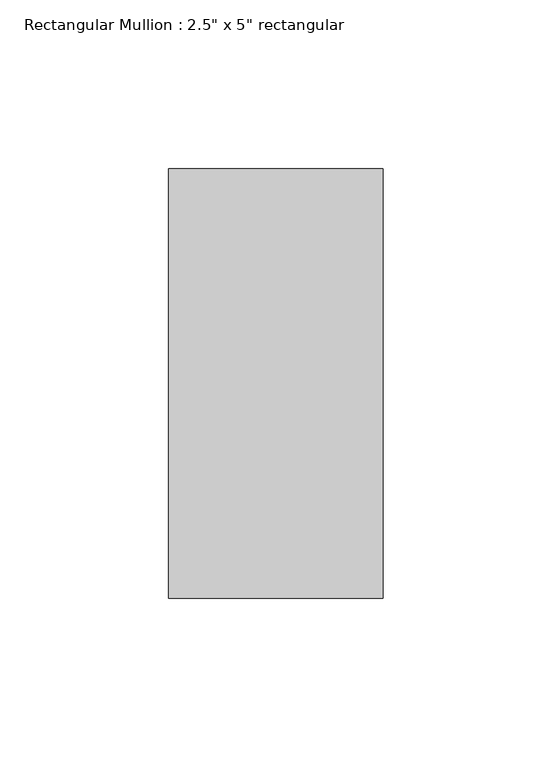
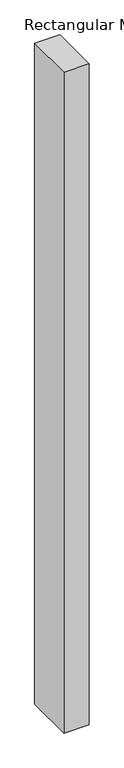
"""IFC4 building model written with IfcOpenShell, lengths in millimetres: member geometry."""

from ifc_helpers import new_model, si_unit, frame, origin, place, context, project, spatial, polyline, outline, extrude, source, transform, mapped, element, save


def member_ef20d1bc(model_context):
    return source(origin(), model_context, "Body", "SweptSolid", [
        extrude(outline(polyline([(0.0, 63.5), (0.0, -63.5), (-63.5, -63.5), (-63.5, 63.5), (0.0, 63.5)])), frame((0.0, 0.0, -1757.093674), z_axis=(0.0, 0.0, 1.0), x_axis=(1.0, 0.0, 0.0)), (0.0, 0.0, 1.0), 1757.093674),
    ])


if __name__ == "__main__":
    model = new_model("IFC4")
    model_context = context("Model", 3, world=origin())
    ifc_project = project(units=[si_unit("LENGTHUNIT", "METRE", prefix="MILLI")], contexts=[model_context])
    site = spatial("IfcSite", under=ifc_project)
    building = spatial("IfcBuilding", under=site)
    placement = place(None, origin())
    member_shape = member_ef20d1bc(model_context)
    element("IfcMember", 1, ObjectType="Rectangular Mullion : 2.5\" x 5\" rectangular", at=placement, inside=building, context=model_context, shape_type="MappedRepresentation", body=[
        mapped(member_shape, transform((0.0, 0.0, 0.0), x_axis=(1.0, 0.0, 0.0), y_axis=(0.0, 1.0, 0.0), z_axis=(0.0, 0.0, 1.0))),
    ])
    save(model, "model.ifc")

# Revit data of these elements
# Type "Rectangular Mullion : 2.5\" x 5\" rectangular"
#   built-in parameter 1007304 = 0.416667 (stored number, unit not read)
#   built-in parameter 1007301 = 0.104167 (stored number, unit not read)
#   built-in parameter 1007300 = 0.104167 (stored number, unit not read)
# Element 1 (IfcMember, "Rectangular Mullion : 2.5\" x 5\" rectangular")
#   Materials on its faces: "Aluminum"
# Materials
#   "Aluminum": class "Metal", colour RGB 247 247 247, transparency 0, Description = "Aluminum 6061", Cost = 0
